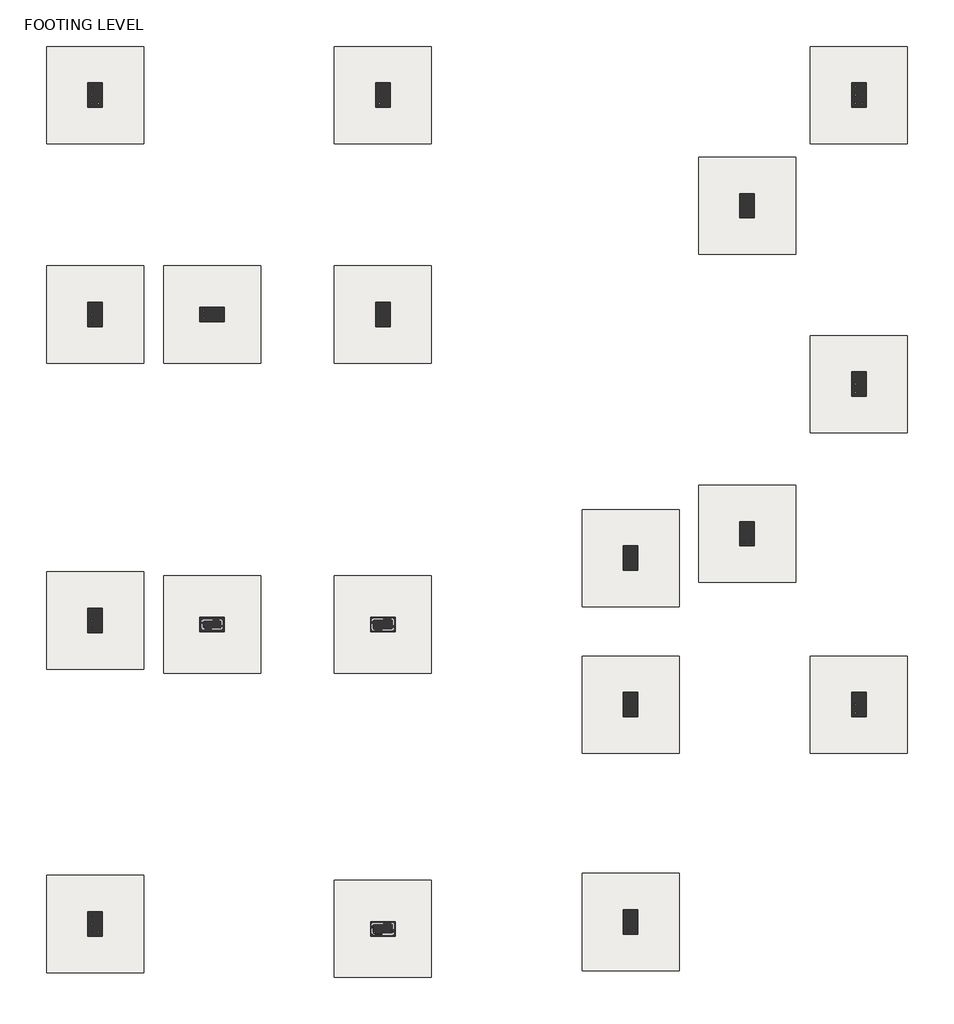
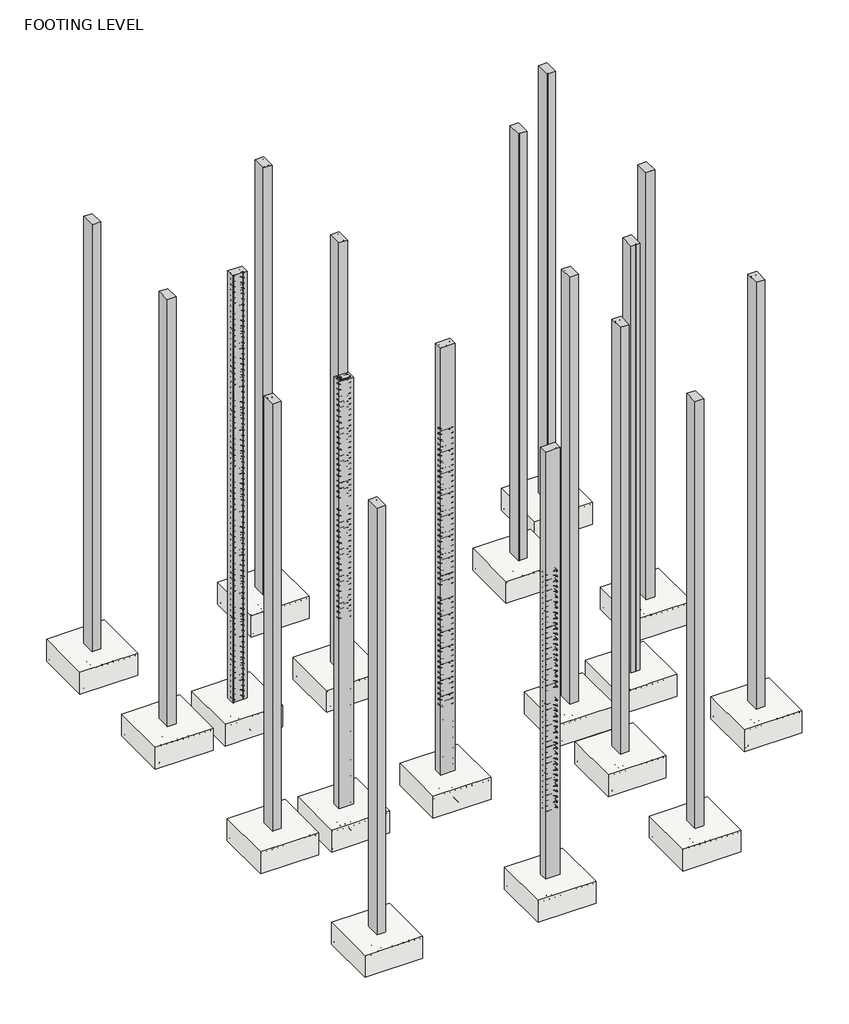
# One storey, part 1 of 10: 18 columns, 18 slabs.
"""IFC4 building model written with IfcOpenShell, lengths in millimetres."""

from ifc_helpers import new_model, si_unit, frame, origin, place, context, project, spatial, polyline, outline, extrude, faceted_brep, transform, mapped, element, save
from components import footing_rectangular_5_c859e583

model = new_model("IFC4")

# Units and contexts
model_context = context("Model", 3, world=origin())
ifc_project = project(units=[si_unit("LENGTHUNIT", "METRE", prefix="MILLI")], contexts=[model_context])

# Site, building, storey
site = spatial("IfcSite", under=ifc_project)
building = spatial("IfcBuilding", under=site)
storey = spatial("IfcBuildingStorey", under=building, Name="FOOTING LEVEL", Elevation=-1371.6)

# Columns
placement = place(None, origin())
element("IfcColumn", 1, ObjectType="Concrete-Rectangular-Column : 1'3\" X 9\"", at=placement, inside=storey, context=model_context, shape_type="SweptSolid", body=[
    extrude(outline(polyline([(-14598.2918223, 420.0576713), (-14598.2918223, 39.0576713), (-14826.8918223, 39.0576713), (-14826.8918223, 420.0576713), (-14598.2918223, 420.0576713)])), frame((0.0, 0.0, -1371.6), z_axis=(0.0, 0.0, 1.0), x_axis=(1.0, 0.0, 0.0)), (0.0, 0.0, 1.0), 11887.2),
])
element("IfcColumn", 2, ObjectType="Concrete-Rectangular-Column : 1'3\" X 9\"", at=placement, inside=storey, context=model_context, shape_type="SweptSolid", body=[
    extrude(outline(polyline([(-6425.8418223, 70.8078802), (-6425.8418223, 451.8078802), (-6197.2418223, 451.8078802), (-6197.2418223, 70.8078802), (-6425.8418223, 70.8078802)])), frame((0.0, 0.0, -1371.6), z_axis=(0.0, 0.0, 1.0), x_axis=(1.0, 0.0, 0.0)), (0.0, 0.0, 1.0), 11887.2),
])
element("IfcColumn", 3, ObjectType="Concrete-Rectangular-Column : 1'3\" X 9\"", at=placement, inside=storey, context=model_context, shape_type="SweptSolid", body=[
    extrude(outline(polyline([(-6425.8418223, 3480.7578802), (-6425.8418223, 3861.7578802), (-6197.2418223, 3861.7578802), (-6197.2418223, 3480.7578802), (-6425.8418223, 3480.7578802)])), frame((0.0, 0.0, -1371.6), z_axis=(0.0, 0.0, 1.0), x_axis=(1.0, 0.0, 0.0)), (0.0, 0.0, 1.0), 11887.2),
])
element("IfcColumn", 4, ObjectType="Concrete-Rectangular-Column : 1'3\" X 9\"", at=placement, inside=storey, context=model_context, shape_type="SweptSolid", body=[
    extrude(outline(polyline([(-2844.4418223, 3480.7578802), (-2844.4418223, 3861.7578802), (-2615.8418223, 3861.7578802), (-2615.8418223, 3480.7578802), (-2844.4418223, 3480.7578802)])), frame((0.0, 0.0, -1371.6), z_axis=(0.0, 0.0, 1.0), x_axis=(1.0, 0.0, 0.0)), (0.0, 0.0, 1.0), 11887.2),
])
element("IfcColumn", 5, ObjectType="Concrete-Rectangular-Column : 1'3\" X 9\"", at=placement, inside=storey, context=model_context, shape_type="SweptSolid", body=[
    extrude(outline(polyline([(-2844.4418223, 8509.9578802), (-2844.4418223, 8890.9578802), (-2615.8418223, 8890.9578802), (-2615.8418223, 8509.9578802), (-2844.4418223, 8509.9578802)])), frame((0.0, 0.0, -1371.6), z_axis=(0.0, 0.0, 1.0), x_axis=(1.0, 0.0, 0.0)), (0.0, 0.0, 1.0), 11887.2),
])
element("IfcColumn", 6, ObjectType="Concrete-Rectangular-Column : 1'3\" X 9\"", at=placement, inside=storey, context=model_context, shape_type="SweptSolid", body=[
    extrude(outline(polyline([(-4597.0418223, 6160.4578802), (-4597.0418223, 6541.4578802), (-4368.4418223, 6541.4578802), (-4368.4418223, 6160.4578802), (-4597.0418223, 6160.4578802)])), frame((0.0, 0.0, -1371.6), z_axis=(0.0, 0.0, 1.0), x_axis=(1.0, 0.0, 0.0)), (0.0, 0.0, 1.0), 11887.2),
])
element("IfcColumn", 7, ObjectType="Concrete-Rectangular-Column : 1'3\" X 9\"", at=placement, inside=storey, context=model_context, shape_type="SweptSolid", body=[
    extrude(outline(polyline([(-6425.8418223, 5779.4578802), (-6425.8418223, 6160.4578802), (-6197.2418223, 6160.4578802), (-6197.2418223, 5779.4578802), (-6425.8418223, 5779.4578802)])), frame((0.0, 0.0, -1371.6), z_axis=(0.0, 0.0, 1.0), x_axis=(1.0, 0.0, 0.0)), (0.0, 0.0, 1.0), 11887.2),
])
element("IfcColumn", 8, ObjectType="Concrete-Rectangular-Column : 1'3\" X 9\"", at=placement, inside=storey, context=model_context, shape_type="SweptSolid", body=[
    extrude(outline(polyline([(-12686.9418223, 4813.8251382), (-13067.9418223, 4813.8251382), (-13067.9418223, 5042.4251382), (-12686.9418223, 5042.4251382), (-12686.9418223, 4813.8251382)])), frame((0.0, 0.0, -1371.6), z_axis=(0.0, 0.0, 1.0), x_axis=(1.0, 0.0, 0.0)), (0.0, 0.0, 1.0), 11887.2),
])
element("IfcColumn", 9, ObjectType="Concrete-Rectangular-Column : 1'3\" X 9\"", at=placement, inside=storey, context=model_context, shape_type="SweptSolid", body=[
    extrude(outline(polyline([(-14598.2918223, 5182.5578802), (-14598.2918223, 4801.5578802), (-14826.8918223, 4801.5578802), (-14826.8918223, 5182.5578802), (-14598.2918223, 5182.5578802)])), frame((0.0, 0.0, -1371.6), z_axis=(0.0, 0.0, 1.0), x_axis=(1.0, 0.0, 0.0)), (0.0, 0.0, 1.0), 11887.2),
])
element("IfcColumn", 10, ObjectType="Concrete-Rectangular-Column : 1'3\" X 9\"", at=placement, inside=storey, context=model_context, shape_type="SweptSolid", body=[
    extrude(outline(polyline([(-10083.4418223, 9983.1578802), (-10083.4418223, 9602.1578802), (-10312.0418223, 9602.1578802), (-10312.0418223, 9983.1578802), (-10083.4418223, 9983.1578802)])), frame((0.0, 0.0, -1371.6), z_axis=(0.0, 0.0, 1.0), x_axis=(1.0, 0.0, 0.0)), (0.0, 0.0, 1.0), 11887.2),
])
element("IfcColumn", 11, ObjectType="Concrete-Rectangular-Column : 1'3\" X 9\"", at=placement, inside=storey, context=model_context, shape_type="SweptSolid", body=[
    extrude(outline(polyline([(-10083.4418223, 13424.8578802), (-10083.4418223, 13043.8578802), (-10312.0418223, 13043.8578802), (-10312.0418223, 13424.8578802), (-10083.4418223, 13424.8578802)])), frame((0.0, 0.0, -1371.6), z_axis=(0.0, 0.0, 1.0), x_axis=(1.0, 0.0, 0.0)), (0.0, 0.0, 1.0), 11887.2),
])
element("IfcColumn", 12, ObjectType="Concrete-Rectangular-Column : 1'3\" X 9\"", at=placement, inside=storey, context=model_context, shape_type="SweptSolid", body=[
    extrude(outline(polyline([(-14598.2918223, 13424.8578802), (-14598.2918223, 13043.8578802), (-14826.8918223, 13043.8578802), (-14826.8918223, 13424.8578802), (-14598.2918223, 13424.8578802)])), frame((0.0, 0.0, -1371.6), z_axis=(0.0, 0.0, 1.0), x_axis=(1.0, 0.0, 0.0)), (0.0, 0.0, 1.0), 11887.2),
])
element("IfcColumn", 13, ObjectType="Concrete-Rectangular-Column : 1'3\" X 9\"", at=placement, inside=storey, context=model_context, shape_type="SweptSolid", body=[
    extrude(outline(polyline([(-4368.4418223, 11687.653797), (-4368.4418223, 11306.653797), (-4597.0418223, 11306.653797), (-4597.0418223, 11687.653797), (-4368.4418223, 11687.653797)])), frame((0.0, 0.0, -1371.6), z_axis=(0.0, 0.0, 1.0), x_axis=(1.0, 0.0, 0.0)), (0.0, 0.0, 1.0), 11887.2),
])
element("IfcColumn", 14, ObjectType="Concrete-Rectangular-Column : 1'3\" X 9\"", at=placement, inside=storey, context=model_context, shape_type="SweptSolid", body=[
    extrude(outline(polyline([(-2615.8418223, 13424.8578802), (-2615.8418223, 13043.8578802), (-2844.4418223, 13043.8578802), (-2844.4418223, 13424.8578802), (-2615.8418223, 13424.8578802)])), frame((0.0, 0.0, -1371.6), z_axis=(0.0, 0.0, 1.0), x_axis=(1.0, 0.0, 0.0)), (0.0, 0.0, 1.0), 11887.2),
])
element("IfcColumn", 15, ObjectType="Concrete-Rectangular-Column : 1'3\" X 9\"", at=placement, inside=storey, context=model_context, shape_type="SweptSolid", body=[
    extrude(outline(polyline([(-13067.9418223, 9906.9578802), (-12686.9418223, 9906.9578802), (-12686.9418223, 9678.3578802), (-13067.9418223, 9678.3578802), (-13067.9418223, 9906.9578802)])), frame((0.0, 0.0, -1371.6), z_axis=(0.0, 0.0, 1.0), x_axis=(1.0, 0.0, 0.0)), (0.0, 0.0, 1.0), 11887.2),
])
element("IfcColumn", 16, ObjectType="Concrete-Rectangular-Column : 1'3\" X 9\"", at=placement, inside=storey, context=model_context, shape_type="SweptSolid", body=[
    extrude(outline(polyline([(-14598.2918223, 9983.1578802), (-14598.2918223, 9602.1578802), (-14826.8918223, 9602.1578802), (-14826.8918223, 9983.1578802), (-14598.2918223, 9983.1578802)])), frame((0.0, 0.0, -1371.6), z_axis=(0.0, 0.0, 1.0), x_axis=(1.0, 0.0, 0.0)), (0.0, 0.0, 1.0), 11887.2),
])
element("IfcColumn", 17, ObjectType="Concrete-Rectangular-Column : 1'3\" X 9\"", at=placement, inside=storey, context=model_context, shape_type="Brep", body=[
    faceted_brep([(-10007.2418223, 4813.8251382, -1371.6), (-10388.2418223, 4813.8251382, -1371.6), (-10388.2418223, 5042.4251382, -1371.6), (-10007.2418223, 5042.4251382, -1371.6), (-10007.2418223, 4813.8251382, 10515.6), (-10388.2418223, 4813.8251382, 10515.6), (-10388.2418223, 4813.8251382, 7010.4), (-10388.2418223, 4813.8251382, 6858.0), (-10388.2418223, 4813.8251382, 3657.6), (-10388.2418223, 4813.8251382, 3505.2), (-10388.2418223, 4813.8251382, 304.8), (-10388.2418223, 4813.8251382, 152.4), (-10007.2418223, 4813.8251382, 152.4), (-10007.2418223, 4813.8251382, 304.8), (-10007.2418223, 4813.8251382, 3505.2), (-10007.2418223, 4813.8251382, 3657.6), (-10007.2418223, 4813.8251382, 6858.0), (-10007.2418223, 4813.8251382, 7010.4), (-10388.2418223, 5042.4251382, 10515.6), (-10388.2418223, 5042.4251382, 7010.4), (-10388.2418223, 5042.4251382, 6858.0), (-10388.2418223, 5042.4251382, 3657.6), (-10388.2418223, 5042.4251382, 3505.2), (-10388.2418223, 5042.4251382, 304.8), (-10388.2418223, 5042.4251382, 152.4), (-10007.2418223, 5042.4251382, 10515.6), (-10007.2418223, 5042.4251382, 7010.4), (-10007.2418223, 5042.4251382, 6858.0), (-10007.2418223, 5042.4251382, 3657.6), (-10007.2418223, 5042.4251382, 3505.2), (-10007.2418223, 5042.4251382, 304.8), (-10007.2418223, 5042.4251382, 152.4)], [[[0, 1, 2, 3]], [[4, 5, 6, 7, 8, 9, 10, 11, 1, 0, 12, 13, 14, 15, 16, 17]], [[5, 18, 19, 20, 21, 22, 23, 24, 2, 1, 11, 10, 9, 8, 7, 6]], [[18, 25, 26, 27, 28, 29, 30, 31, 3, 2, 24, 23, 22, 21, 20, 19]], [[25, 4, 17, 16, 15, 14, 13, 12, 0, 3, 31, 30, 29, 28, 27, 26]], [[4, 25, 18, 5]]]),
])
element("IfcColumn", 18, ObjectType="Concrete-Rectangular-Column : 1'3\" X 9\"", at=placement, inside=storey, context=model_context, shape_type="Brep", body=[
    faceted_brep([(-10388.2418223, 267.6576713, -1371.6), (-10007.2418223, 267.6576713, -1371.6), (-10007.2418223, 39.0576713, -1371.6), (-10388.2418223, 39.0576713, -1371.6), (-10388.2418223, 267.6576713, 10515.6), (-10007.2418223, 267.6576713, 10515.6), (-10007.2418223, 267.6576713, 304.8), (-10007.2418223, 267.6576713, 152.4), (-10007.2418223, 39.0576713, 10515.6), (-10007.2418223, 39.0576713, 457.2), (-10007.2418223, 39.0576713, 152.4), (-10388.2418223, 39.0576713, 10515.6)], [[[0, 1, 2, 3]], [[4, 5, 6, 7, 1, 0]], [[5, 8, 9, 10, 2, 1, 7, 6]], [[8, 11, 3, 2, 10, 9]], [[11, 4, 0, 3]], [[4, 11, 8, 5]]]),
])

# Slabs
footing_rectangular_5_shape = footing_rectangular_5_c859e583(model_context)
element("IfcSlab", 19, ObjectType="Footing-Rectangular : 5'", at=placement, inside=storey, context=model_context, shape_type="MappedRepresentation", body=[
    mapped(footing_rectangular_5_shape, transform((-6311.5418223, 261.3078802, -1371.6), x_axis=(-1.0, 0.0, 0.0), y_axis=(0.0, -1.0, 0.0), z_axis=(0.0, 0.0, 1.0))),
])
element("IfcSlab", 20, ObjectType="Footing-Rectangular : 5'", at=placement, inside=storey, context=model_context, shape_type="MappedRepresentation", body=[
    mapped(footing_rectangular_5_shape, transform((-6311.5418223, 3671.2578802, -1371.6), x_axis=(-1.0, 0.0, 0.0), y_axis=(0.0, -1.0, 0.0), z_axis=(0.0, 0.0, 1.0))),
])
element("IfcSlab", 21, ObjectType="Footing-Rectangular : 5'", at=placement, inside=storey, context=model_context, shape_type="MappedRepresentation", body=[
    mapped(footing_rectangular_5_shape, transform((-2730.1418223, 3671.2578802, -1371.6), x_axis=(-1.0, 0.0, 0.0), y_axis=(0.0, -1.0, 0.0), z_axis=(0.0, 0.0, 1.0))),
])
element("IfcSlab", 22, ObjectType="Footing-Rectangular : 5'", at=placement, inside=storey, context=model_context, shape_type="MappedRepresentation", body=[
    mapped(footing_rectangular_5_shape, transform((-2730.1418223, 8700.4578802, -1371.6), x_axis=(-1.0, 0.0, 0.0), y_axis=(0.0, -1.0, 0.0), z_axis=(0.0, 0.0, 1.0))),
])
element("IfcSlab", 23, ObjectType="Footing-Rectangular : 5'", at=placement, inside=storey, context=model_context, shape_type="MappedRepresentation", body=[
    mapped(footing_rectangular_5_shape, transform((-4482.7418223, 6350.9578802, -1371.6), x_axis=(-1.0, 0.0, 0.0), y_axis=(0.0, -1.0, 0.0), z_axis=(0.0, 0.0, 1.0))),
])
element("IfcSlab", 24, ObjectType="Footing-Rectangular : 5'", at=placement, inside=storey, context=model_context, shape_type="MappedRepresentation", body=[
    mapped(footing_rectangular_5_shape, transform((-6311.5418223, 5969.9578802, -1371.6), x_axis=(-1.0, 0.0, 0.0), y_axis=(0.0, -1.0, 0.0), z_axis=(0.0, 0.0, 1.0))),
])
element("IfcSlab", 25, ObjectType="Footing-Rectangular : 5'", at=placement, inside=storey, context=model_context, shape_type="MappedRepresentation", body=[
    mapped(footing_rectangular_5_shape, transform((-12877.4418223, 4928.1251382, -1371.6), x_axis=(0.0, -1.0, 0.0), y_axis=(1.0, 0.0, 0.0), z_axis=(0.0, 0.0, 1.0))),
])
element("IfcSlab", 26, ObjectType="Footing-Rectangular : 5'", at=placement, inside=storey, context=model_context, shape_type="MappedRepresentation", body=[
    mapped(footing_rectangular_5_shape, transform((-14712.5918223, 4992.0578802, -1371.6), x_axis=(1.0, 0.0, 0.0), y_axis=(0.0, 1.0, 0.0), z_axis=(0.0, 0.0, 1.0))),
])
element("IfcSlab", 27, ObjectType="Footing-Rectangular : 5'", at=placement, inside=storey, context=model_context, shape_type="MappedRepresentation", body=[
    mapped(footing_rectangular_5_shape, transform((-10197.7418223, 9792.6578802, -1371.6), x_axis=(1.0, 0.0, 0.0), y_axis=(0.0, 1.0, 0.0), z_axis=(0.0, 0.0, 1.0))),
])
element("IfcSlab", 28, ObjectType="Footing-Rectangular : 5'", at=placement, inside=storey, context=model_context, shape_type="MappedRepresentation", body=[
    mapped(footing_rectangular_5_shape, transform((-10197.7418223, 13234.3578802, -1371.6), x_axis=(1.0, 0.0, 0.0), y_axis=(0.0, 1.0, 0.0), z_axis=(0.0, 0.0, 1.0))),
])
element("IfcSlab", 29, ObjectType="Footing-Rectangular : 5'", at=placement, inside=storey, context=model_context, shape_type="MappedRepresentation", body=[
    mapped(footing_rectangular_5_shape, transform((-14712.5918223, 13234.3578802, -1371.6), x_axis=(1.0, 0.0, 0.0), y_axis=(0.0, 1.0, 0.0), z_axis=(0.0, 0.0, 1.0))),
])
element("IfcSlab", 30, ObjectType="Footing-Rectangular : 5'", at=placement, inside=storey, context=model_context, shape_type="MappedRepresentation", body=[
    mapped(footing_rectangular_5_shape, transform((-4482.7418223, 11497.153797, -1371.6), x_axis=(1.0, 0.0, 0.0), y_axis=(0.0, 1.0, 0.0), z_axis=(0.0, 0.0, 1.0))),
])
element("IfcSlab", 31, ObjectType="Footing-Rectangular : 5'", at=placement, inside=storey, context=model_context, shape_type="MappedRepresentation", body=[
    mapped(footing_rectangular_5_shape, transform((-2730.1418223, 13234.3578802, -1371.6), x_axis=(1.0, 0.0, 0.0), y_axis=(0.0, 1.0, 0.0), z_axis=(0.0, 0.0, 1.0))),
])
element("IfcSlab", 32, ObjectType="Footing-Rectangular : 5'", at=placement, inside=storey, context=model_context, shape_type="MappedRepresentation", body=[
    mapped(footing_rectangular_5_shape, transform((-14712.5918223, 229.5576713, -1371.6), x_axis=(1.0, 0.0, 0.0), y_axis=(0.0, 1.0, 0.0), z_axis=(0.0, 0.0, 1.0))),
])
element("IfcSlab", 33, ObjectType="Footing-Rectangular : 5'", at=placement, inside=storey, context=model_context, shape_type="MappedRepresentation", body=[
    mapped(footing_rectangular_5_shape, transform((-12877.4418223, 9792.6578802, -1371.6), x_axis=(0.0, 1.0, 0.0), y_axis=(-1.0, 0.0, 0.0), z_axis=(0.0, 0.0, 1.0))),
])
element("IfcSlab", 34, ObjectType="Footing-Rectangular : 5'", at=placement, inside=storey, context=model_context, shape_type="MappedRepresentation", body=[
    mapped(footing_rectangular_5_shape, transform((-14712.5918223, 9792.6578802, -1371.6), x_axis=(1.0, 0.0, 0.0), y_axis=(0.0, 1.0, 0.0), z_axis=(0.0, 0.0, 1.0))),
])
element("IfcSlab", 35, ObjectType="Footing-Rectangular : 5'", at=placement, inside=storey, context=model_context, shape_type="MappedRepresentation", body=[
    mapped(footing_rectangular_5_shape, transform((-10197.7418223, 4928.1251382, -1371.6), x_axis=(0.0, -1.0, 0.0), y_axis=(1.0, 0.0, 0.0), z_axis=(0.0, 0.0, 1.0))),
])
element("IfcSlab", 36, ObjectType="Footing-Rectangular : 5'", at=placement, inside=storey, context=model_context, shape_type="MappedRepresentation", body=[
    mapped(footing_rectangular_5_shape, transform((-10197.7418223, 153.3576713, -1371.6), x_axis=(0.0, 1.0, 0.0), y_axis=(-1.0, 0.0, 0.0), z_axis=(0.0, 0.0, 1.0))),
])

save(model, "model.ifc")

# Revit data of these elements
# Type "Concrete-Rectangular-Column : 1'3\" X 9\""
#   Assembly Code = "B10"
#   b = 0' - 9"
#   h = 1' - 3"
#   Structural Material [instance default] = Concrete, Cast-in-Place gray
# Type "Footing-Rectangular : 5'"
#   Assembly Code = "A1010100"
#   Width = 5' - 0"
#   Length = 5' - 0"
#   Foundation Thickness = 2' - 0"
#   Structural Material [instance default] = Concrete, Cast-in-Place gray
# Elements 1, 2, 3, 4, 5, 6, 7, 8, 9, 10, 11, 12, 13, 14, 15, 16, 17, 18 (IfcColumn, "Concrete-Rectangular-Column : 1'3\" X 9\"")
#   Structural Material = Concrete, Cast-in-Place gray
#   Phase Created = New Construction
#   Materials on its faces: "Concrete, Cast-in-Place gray"
# Elements 19, 20, 21, 22, 23, 24, 25, 26, 27, 28, 29, 30, 31, 32, 33, 34, 35, 36 (IfcSlab, "Footing-Rectangular : 5'")
#   Structural Material = Concrete, Cast-in-Place gray
#   Phase Created = New Construction
#   Materials on its faces: "Concrete, Cast-in-Place gray"
# Materials
#   "Concrete, Cast-in-Place gray": class "Concrete", colour RGB 192 192 192, transparency 0, Description = "Cast-in-place concrete", Cost = 0
